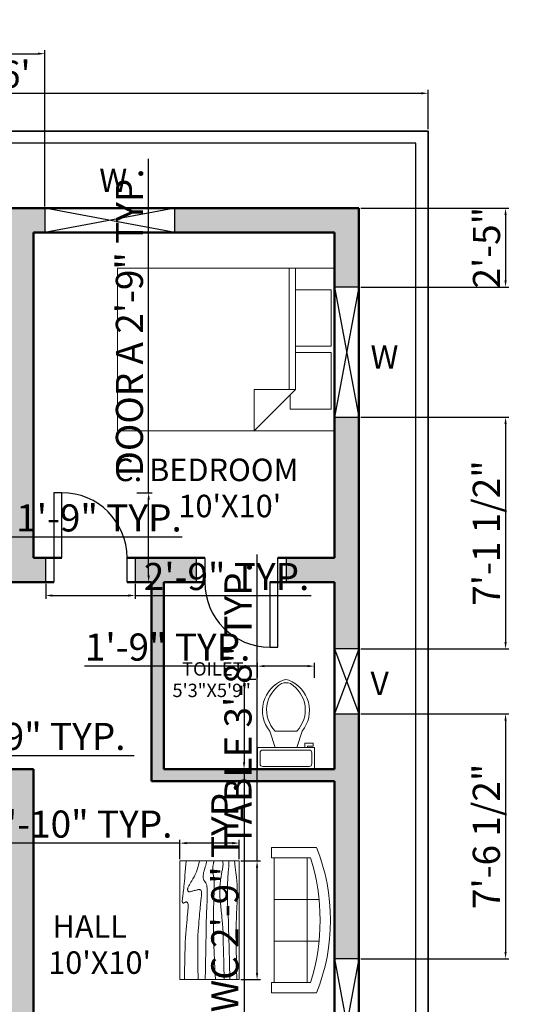
# Model space of a CAD drawing. Units: inches. Extents: x 2789 to 3623, y 2388 to 2993.
# Tile 5 of 5: x 3435 to 3623, y 2601 to 2964. Entities that reach past the tile are written whole.
import ezdxf

# ---------------------------------------------------------------- set-up
doc = ezdxf.new("R2010")
doc.units = ezdxf.units.IN
for name, color, linetype, lineweight in [('A-ANNO-DIMS', 2, 'Continuous', 18), ('A-ANNO-TEXT', 7, 'Continuous', 18), ('A-AREA-IDEN', 7, 'Continuous', 18), ('A-FLOR-FIXT', 9, 'Continuous', 18), ('A-FURN', 8, 'Continuous', 18), ('A-WALL', 7, 'Continuous', 50), ('A-WALL-PATT', 5, 'Continuous', 13), ('C-PROP', 7, 'Continuous', 35), ('d', 1, 'Continuous', 25), ('L-WALL', 7, 'Continuous', 25), ('v', 6, 'Continuous', 25), ('w', 170, 'Continuous', 25)]:
    doc.layers.add(name, color=color, linetype=linetype, lineweight=lineweight)
doc.styles.get("Standard").update_dxf_attribs({"font": 'arial.ttf'})
doc.dimstyles.new('ISO-25', dxfattribs={"dimtxt": 10, "dimasz": 2.5, "dimexe": 1.25, "dimexo": 0.625, "dimtad": 1, "dimlunit": 4, "dimtxsty": 'Standard', "dimcen": 2.5, "dimadec": 0, "dimazin": 0, "dimtfac": 1, "dimtmove": 0, "dimatfit": 3, "dimfxl": 1, "dimarcsym": 0})

# ---------------------------------------------------------------- blocks, each defined once
blk = doc.blocks.new('Sofa - Roundback 7 ft.')
for p, q in [((-12.00002, -32.4421), (-12.00003, -6.5971)), ((11.99997, -32.4421), (11.99998, -6.5971)), ((-36.000027, -34), (-36.000027, -11.4696)), ((-35.999844, -13.3819), (35.9998, -13.3819)), ((35.99998, -34), (35.99998, -11.4696)), ((-36.000027, -32.4421), (35.99998, -32.4421))]:
    blk.add_line(p, q)
for points in [[(-36.000027, -34), (-42.000027, -34), (-42.000027, -8)], [(41.99998, -8), (41.99998, -34), (35.99998, -34)]]:
    blk.add_lwpolyline(points)
for centre, radius, start, end in [((0, -114.25), 114.25, 68.43141, 111.5686), ((-0.00001, -127.1968), 121.1968, 72.72033, 107.2797)]:
    blk.add_arc(centre, radius, start, end)
blk = doc.blocks.new('Table - Rectangular Woodgrain 60 x 30 in.')
for p, q in [((0, 0), (0, -30)), ((60, 0), (0, 0)), ((60, -30), (60, 0)), ((0, -30), (60, -30))]:
    blk.add_line(p, q)
for points in [[(0, -2.4), (4.8155, -2.418), (9.0302, -2.4688), (12.709, -2.5477), (15.9167, -2.65), (18.7181, -2.7711), (21.1781, -2.9063), (23.3616, -3.0508), (25.3333, -3.2), (27.1477, -3.3495), (28.8172, -3.4958), (30.3437, -3.636), (31.7291, -3.7667), (32.9756, -3.8849), (34.0849, -3.9875), (35.059, -4.0714), (35.9, -4.1334), (36.6114, -4.1711), (37.2041, -4.1854), (37.6906, -4.1779), (38.0833, -4.15), (38.3948, -4.1034), (38.6375, -4.0396), (38.8239, -3.9602), (38.9666, -3.8667), (39.0764, -3.7608), (39.1573, -3.6448), (39.2116, -3.521), (39.2416, -3.3917), (39.2498, -3.2593), (39.2385, -3.1261), (39.21, -2.9944), (39.1666, -2.8667), (39.111, -2.7447), (39.0468, -2.6281), (38.978, -2.5163), (38.9083, -2.4083), (38.8418, -2.3035), (38.7823, -2.201), (38.7337, -2.1001), (38.7, -2), (38.6844, -1.9003), (38.6875, -1.8021), (38.7094, -1.707), (38.75, -1.6167), (38.8094, -1.5326), (38.8875, -1.4563), (38.9844, -1.3893), (39.1, -1.3333), (39.2351, -1.2896), (39.3937, -1.2583), (39.5804, -1.2396), (39.8, -1.2333), (40.057, -1.2396), (40.3562, -1.2583), (40.7023, -1.2896), (41.1, -1.3333), (41.5547, -1.3895), (42.0755, -1.4573), (42.6721, -1.5361), (43.3542, -1.625), (44.1316, -1.7233), (45.014, -1.8302), (46.0114, -1.9449), (47.1333, -2.0667), (48.3862, -2.1947), (49.7625, -2.3281), (51.2513, -2.4663), (52.8416, -2.6083), (54.5226, -2.7535), (56.2833, -2.9011), (58.1127, -3.0501), (60, -3.2)], [(0, -9.2), (6.5759, -9.0858), (11.9385, -9.0365), (16.2527, -9.0418), (19.6833, -9.0917), (22.3952, -9.1759), (24.5531, -9.2844), (26.322, -9.4069), (27.8666, -9.5333), (29.3241, -9.6553), (30.7203, -9.7719), (32.0532, -9.8837), (33.3208, -9.9917), (34.5213, -10.0965), (35.6526, -10.199), (36.7128, -10.2999), (37.7, -10.4), (38.6129, -10.4996), (39.4531, -10.5969), (40.223, -10.6895), (40.925, -10.775), (41.5613, -10.8512), (42.1344, -10.9156), (42.6465, -10.966), (43.1, -11), (43.4976, -11.0158), (43.8437, -11.0136), (44.143, -10.9942), (44.4, -10.9583), (44.6195, -10.9069), (44.8062, -10.8406), (44.9648, -10.7603), (45.1, -10.6667), (45.2155, -10.5598), (45.3114, -10.4365), (45.3871, -10.2929), (45.4416, -10.125), (45.4743, -9.929), (45.4844, -9.7011), (45.4709, -9.4371), (45.4333, -9.1333), (45.3716, -8.7883), (45.2896, -8.4104), (45.1919, -8.0107), (45.0833, -7.6), (44.9685, -7.1893), (44.8521, -6.7896), (44.7388, -6.4117), (44.6333, -6.0667), (44.54, -5.7628), (44.4614, -5.4979), (44.4001, -5.2675), (44.3583, -5.0667), (44.3384, -4.8909), (44.3427, -4.7354), (44.3736, -4.5956), (44.4333, -4.4667), (44.5236, -4.3453), (44.6427, -4.2333), (44.7884, -4.1339), (44.9583, -4.05), (45.1501, -3.9849), (45.3614, -3.9417), (45.59, -3.9234), (45.8333, -3.9333), (46.0915, -3.9749), (46.3734, -4.0531), (46.6906, -4.1736), (47.0542, -4.3417), (47.4756, -4.5629), (47.9661, -4.8427), (48.5372, -5.1866), (49.2, -5.6), (49.9676, -6.0844), (50.8594, -6.625), (51.8965, -7.2031), (53.1, -7.8), (54.491, -8.3969), (56.0906, -8.975), (57.9199, -9.5156), (60, -10)], [(0, -12.8), (5.1847, -12.9322), (9.6213, -13.0323), (13.3963, -13.1059), (16.5958, -13.1583), (19.3063, -13.1952), (21.614, -13.2219), (23.6054, -13.2439), (25.3666, -13.2667), (26.9728, -13.2947), (28.4531, -13.3281), (29.8256, -13.3663), (31.1083, -13.4083), (32.3191, -13.4535), (33.476, -13.501), (34.597, -13.5501), (35.7, -13.6), (36.7984, -13.6497), (37.8875, -13.6979), (38.9578, -13.743), (40, -13.7833), (41.0047, -13.8174), (41.9625, -13.8438), (42.864, -13.8607), (43.7, -13.8667), (44.4631, -13.8604), (45.1552, -13.8417), (45.7801, -13.8104), (46.3416, -13.7667), (46.8439, -13.7104), (47.2906, -13.6417), (47.6858, -13.5604), (48.0333, -13.4667), (48.3375, -13.3608), (48.6042, -13.2448), (48.8396, -13.121), (49.05, -12.9917), (49.2417, -12.8593), (49.4208, -12.7261), (49.5937, -12.5944), (49.7667, -12.4667), (49.9452, -12.3451), (50.1323, -12.2313), (50.3303, -12.1268), (50.5416, -12.0333), (50.7686, -11.9524), (51.0135, -11.8854), (51.2788, -11.8341), (51.5666, -11.8), (51.8785, -11.7843), (52.2116, -11.7865), (52.562, -11.8059), (52.926, -11.8417), (53.2998, -11.8931), (53.6795, -11.9594), (54.0614, -12.0397), (54.4416, -12.1333), (54.8223, -12.2401), (55.2293, -12.3625), (55.6942, -12.5037), (56.2489, -12.6667), (56.9251, -12.8547), (57.7545, -13.0708), (58.7689, -13.3182), (60, -13.6)], [(0, -18), (5.124, -17.7273), (9.6609, -17.5057), (13.6705, -17.3303), (17.2125, -17.1958), (20.3467, -17.0973), (23.1328, -17.0297), (25.6307, -16.9878), (27.9, -16.9667), (29.9928, -16.9617), (31.9302, -16.9703), (33.7254, -16.9907), (35.3917, -17.0208), (36.9423, -17.0588), (38.3906, -17.1026), (39.7499, -17.1503), (41.0333, -17.2), (42.2519, -17.2496), (43.4073, -17.2969), (44.4986, -17.3395), (45.525, -17.375), (46.4858, -17.4012), (47.3802, -17.4156), (48.2074, -17.416), (48.9667, -17.4), (49.6583, -17.3662), (50.2872, -17.3167), (50.8595, -17.2547), (51.3812, -17.1833), (51.8584, -17.1057), (52.2971, -17.025), (52.7034, -16.9443), (53.0833, -16.8667), (53.443, -16.7951), (53.789, -16.7313), (54.128, -16.6768), (54.4666, -16.6334), (54.8115, -16.6024), (55.1693, -16.5854), (55.5465, -16.5841), (55.95, -16.6), (56.3828, -16.6337), (56.8346, -16.6823), (57.2915, -16.7418), (57.7396, -16.8084), (58.165, -16.878), (58.5539, -16.9469), (58.8924, -17.0111), (59.1666, -17.0667), (59.3679, -17.1107), (59.5078, -17.1438), (59.6032, -17.1675), (59.6708, -17.1833), (59.7275, -17.193), (59.7901, -17.1979), (59.8753, -17.1998), (60, -17.2)], [(0, -22.4), (8.0098, -22.2501), (14.4094, -22.1011), (19.4168, -21.9535), (23.25, -21.8083), (26.1269, -21.6663), (28.2656, -21.5281), (29.884, -21.3947), (31.2, -21.2667), (32.3967, -21.1448), (33.5172, -21.0292), (34.5697, -20.9198), (35.5625, -20.8167), (36.5037, -20.7198), (37.4015, -20.6292), (38.2642, -20.5448), (39.1, -20.4667), (39.9164, -20.3951), (40.7187, -20.3313), (41.5117, -20.2768), (42.3, -20.2333), (43.0883, -20.2024), (43.8812, -20.1854), (44.6836, -20.1841), (45.5, -20.2), (46.3328, -20.234), (47.1747, -20.2844), (48.0163, -20.3488), (48.8479, -20.425), (49.66, -20.5106), (50.4429, -20.6031), (51.1872, -20.7004), (51.8833, -20.8), (52.5246, -20.8999), (53.1166, -20.9995), (53.6681, -21.0983), (54.1875, -21.1958), (54.6834, -21.2919), (55.1646, -21.3859), (55.6394, -21.4777), (56.1167, -21.5667), (56.6028, -21.6515), (57.0961, -21.7266), (57.5929, -21.7852), (58.0896, -21.8208), (58.5823, -21.8268), (59.0674, -21.7964), (59.5412, -21.723), (60, -21.6)], [(0, -25.2), (8.6355, -25.0504), (15.7026, -24.9031), (21.4049, -24.7606), (25.9458, -24.625), (29.529, -24.4988), (32.3578, -24.3844), (34.6359, -24.284), (36.5667, -24.2), (38.3213, -24.1341), (39.9417, -24.0854), (41.437, -24.0523), (42.8167, -24.0333), (44.0901, -24.0268), (45.2667, -24.0313), (46.3557, -24.0451), (47.3667, -24.0667), (48.309, -24.0947), (49.1928, -24.1287), (50.0284, -24.168), (50.826, -24.2125), (51.5959, -24.2617), (52.3483, -24.3151), (53.0935, -24.3725), (53.8417, -24.4334), (54.6009, -24.497), (55.3699, -24.561), (56.1454, -24.6226), (56.9239, -24.6792), (57.7021, -24.7279), (58.4764, -24.7662), (59.2435, -24.7911), (60, -24.8)], [(0, -28.8), (5.6867, -28.6681), (10.45, -28.5698), (14.407, -28.5012), (17.675, -28.4584), (20.3711, -28.4374), (22.6125, -28.4344), (24.5164, -28.4455), (26.2, -28.4667), (27.762, -28.4947), (29.2276, -28.5281), (30.6033, -28.5663), (31.8958, -28.6084), (33.1118, -28.6535), (34.2578, -28.7011), (35.3405, -28.7501), (36.3666, -28.8), (37.3443, -28.8497), (38.288, -28.8974), (39.2137, -28.9412), (40.1375, -28.9792), (41.0753, -29.0093), (42.0432, -29.0297), (43.0572, -29.0384), (44.1333, -29.0333), (45.2936, -29.0114), (46.5843, -28.9641), (48.0579, -28.8816), (49.7666, -28.7542), (51.7629, -28.5721), (54.0989, -28.3255), (56.8272, -28.0048), (60, -27.6)]]:
    blk.add_lwpolyline(points)
blk = doc.blocks.new('Toilet - top')
for p, q in [((9.5, -6), (9.5, -2)), ((-10, -8.5), (-8, -8.5)), ((-10, -9.5), (-10, -8.5)), ((-7, -9.5), (-10, -9.5)), ((-8, -8.5), (-8, -8)), ((-7, -8), (-7, -9.5)), ((-4, -8), (-6, -14)), ((4, -8), (6, -14)), ((4, -14), (-4, -14))]:
    blk.add_line(p, q)
blk.add_lwpolyline([(10.5, -8), (10.5, 0), (-10.5, 0), (-10.5, -8)], close=True)
for points in [[(-9.5, -2), (-9.5, -6)], [(8.5, -1), (-8.5, -1)], [(-8.5, -7), (8.5, -7)]]:
    blk.add_lwpolyline(points)
for centre, radius, start, end in [((-8.62, -1.88), 0.884, 81.8699, 188.1301), ((8.62, -1.88), 0.884, 351.8699, 98.1301), ((-8.62, -6.12), 0.884, 171.8699, 278.1301), ((8.62, -6.12), 0.884, 261.8699, 8.1301), ((3.52, -21.58), 12.17, 141.4691, 247.9714), ((4.2, -21.82), 11.33, 136.3677, 238.9468), ((-3.52, -21.58), 12.17, 292.0284, 38.5307), ((-4.2, -21.82), 11.33, 301.053, 43.6321), ((0, -27.88), 4, 245.7318, 294.2682), ((0, -29), 4, 254.8605, 285.1395)]:
    blk.add_arc(centre, radius, start, end)
blk = doc.blocks.new('Bed - Queen')
for p, q in [((0, -80.00003), (0, 0)), ((0, 0), (59.99999, 0)), ((59.99999, 0), (59.99999, -80.00003)), ((7.99999, -1.2), (28.79998, -1.2)), ((7.99999, -14.4), (7.99999, -1.2)), ((28.79998, -1.2), (28.79998, -14.4)), ((31.19999, -1.2), (51.99999, -1.2)), ((31.19999, -14.4), (31.19999, -1.2)), ((51.99999, -1.2), (51.99999, -16.4)), ((0, -14.4), (44.8, -14.4)), ((59.99999, -29.6), (44.8, -14.4)), ((44.8, -14.4), (44.8, -29.6)), ((44.8, -16.8), (0, -16.8)), ((51.99999, -16.4), (46.79936, -16.4)), ((44.8, -29.6), (59.99999, -29.6)), ((59.99999, -80.00003), (0, -80.00003))]:
    blk.add_line(p, q)
blk = doc.blocks.new('*D14')
at = {"layer": 'A-ANNO-DIMS', "color": 0, "lineweight": -2, "transparency": 16777216}
for p, q in [((3273.51, 2923.47), (3273.51, 2938.03)), ((3276.01, 2936.78), (3583.01, 2936.78)), ((3585.51, 2923.47), (3585.51, 2938.03))]:
    blk.add_line(p, q, dxfattribs=at)
at = {"layer": 'A-ANNO-DIMS', "color": 0, "transparency": 16777216}
for points in [[(3276.01, 2937.19), (3276.01, 2936.36), (3273.51, 2936.78)], [(3583.01, 2937.19), (3583.01, 2936.36), (3585.51, 2936.78)]]:
    blk.add_solid(points, dxfattribs=at)
at = {"layer": 'Defpoints', "color": 0, "transparency": 16777216}
for p in [(3585.51, 2936.78), (3273.51, 2922.84), (3585.51, 2922.84)]:
    blk.add_point(p, dxfattribs=at)
at = {"layer": 'A-ANNO-DIMS', "color": 0, "transparency": 16777216, "insert": (3429.51, 2942.51), "char_height": 10, "attachment_point": 5}
blk.add_mtext("26'", dxfattribs=at)
blk = doc.blocks.new('DOOR-24IN-JAMB-9IN')
for points in [[(0, 24), (-3, 24), (-3, 0), (0, 0)], [(-6, 0), (-3, 0), (-3, -9), (-6, -9)], [(24, 0), (27, 0), (27, -9), (24, -9)]]:
    blk.add_lwpolyline(points, close=True)
blk.add_arc((0, 0), 24, 0, 90)
blk = doc.blocks.new('WINDOW-48IN')
for p, q in [((48, 9), (0, 0)), ((48, 0), (0, 9))]:
    blk.add_line(p, q)
blk.add_lwpolyline([(0, 9), (0, 0), (48, 0), (48, 9)], close=True)
blk = doc.blocks.new('VENT-24IN')
for p, q in [((0, 24), (9, 0)), ((9, 24), (0, 0))]:
    blk.add_line(p, q)
blk.add_lwpolyline([(0, 0), (9, 0), (9, 24), (0, 24)], close=True)
blk = doc.blocks.new('*D22')
at = {"layer": 'A-ANNO-DIMS', "color": 0, "lineweight": -2, "transparency": 16777216}
for p, q in [((3482.46, 2789.34), (3482.46, 2912.54)), ((3478.13, 2789.34), (3483.71, 2789.34)), ((3482.46, 2758.84), (3482.46, 2786.84)), ((3478.13, 2756.34), (3483.71, 2756.34))]:
    blk.add_line(p, q, dxfattribs=at)
at = {"layer": 'A-ANNO-DIMS', "color": 0, "transparency": 16777216}
for points in [[(3482.04, 2786.84), (3482.87, 2786.84), (3482.46, 2789.34)], [(3482.04, 2758.84), (3482.87, 2758.84), (3482.46, 2756.34)]]:
    blk.add_solid(points, dxfattribs=at)
at = {"layer": 'Defpoints', "color": 0, "transparency": 16777216}
for p in [(3477.51, 2789.34), (3482.46, 2789.34), (3477.51, 2756.34)]:
    blk.add_point(p, dxfattribs=at)
at = {"layer": 'A-ANNO-DIMS', "color": 0, "transparency": 16777216, "insert": (3476.66, 2852.19), "char_height": 10, "attachment_point": 5, "rotation": 90}
blk.add_mtext('DOOR A 2\'-9" TYP.', dxfattribs=at)
blk = doc.blocks.new('*D23')
at = {"layer": 'A-ANNO-DIMS', "color": 0, "lineweight": -2, "transparency": 16777216}
for p, q in [((3444.51, 2755.72), (3444.51, 2750.14)), ((3477.51, 2755.72), (3477.51, 2750.14)), ((3447.01, 2751.39), (3475.01, 2751.39)), ((3477.51, 2751.39), (3542.38, 2751.39))]:
    blk.add_line(p, q, dxfattribs=at)
at = {"layer": 'A-ANNO-DIMS', "color": 0, "transparency": 16777216}
for points in [[(3447.01, 2751.81), (3447.01, 2750.98), (3444.51, 2751.39)], [(3475.01, 2751.81), (3475.01, 2750.98), (3477.51, 2751.39)]]:
    blk.add_solid(points, dxfattribs=at)
at = {"layer": 'Defpoints', "color": 0, "transparency": 16777216}
for p in [(3444.51, 2756.34), (3477.51, 2756.34), (3477.51, 2751.39)]:
    blk.add_point(p, dxfattribs=at)
at = {"layer": 'A-ANNO-DIMS', "color": 0, "transparency": 16777216, "insert": (3511.19, 2757.12), "char_height": 10, "attachment_point": 5}
blk.add_mtext('2\'-9" TYP.', dxfattribs=at)
blk = doc.blocks.new('*D31')
at = {"layer": 'A-ANNO-DIMS', "color": 0, "lineweight": -2, "transparency": 16777216}
for p, q in [((3410.01, 2777.79), (3410.01, 2771.76)), ((3431.01, 2777.79), (3431.01, 2771.76)), ((3412.51, 2773.01), (3428.51, 2773.01)), ((3431.01, 2773.01), (3494.78, 2773.01))]:
    blk.add_line(p, q, dxfattribs=at)
at = {"layer": 'A-ANNO-DIMS', "color": 0, "transparency": 16777216}
for points in [[(3412.51, 2773.43), (3412.51, 2772.59), (3410.01, 2773.01)], [(3428.51, 2773.43), (3428.51, 2772.59), (3431.01, 2773.01)]]:
    blk.add_solid(points, dxfattribs=at)
at = {"layer": 'Defpoints', "color": 0, "transparency": 16777216}
for p in [(3410.01, 2778.41), (3431.01, 2778.41), (3431.01, 2773.01)]:
    blk.add_point(p, dxfattribs=at)
at = {"layer": 'A-ANNO-DIMS', "color": 0, "transparency": 16777216, "insert": (3464.15, 2778.74), "char_height": 10, "attachment_point": 5}
blk.add_mtext('1\'-9" TYP.', dxfattribs=at)
blk = doc.blocks.new('*D34')
at = {"layer": 'A-ANNO-DIMS', "color": 0, "lineweight": -2, "transparency": 16777216}
for p, q in [((3522.44, 2653.44), (3522.44, 2766.54)), ((3516.49, 2653.44), (3523.69, 2653.44)), ((3522.44, 2612.13), (3522.44, 2650.94)), ((3516.49, 2609.63), (3523.69, 2609.63))]:
    blk.add_line(p, q, dxfattribs=at)
at = {"layer": 'A-ANNO-DIMS', "color": 0, "transparency": 16777216}
for points in [[(3522.02, 2650.94), (3522.85, 2650.94), (3522.44, 2653.44)], [(3522.02, 2612.13), (3522.85, 2612.13), (3522.44, 2609.63)]]:
    blk.add_solid(points, dxfattribs=at)
at = {"layer": 'Defpoints', "color": 0, "transparency": 16777216}
for p in [(3515.86, 2653.44), (3522.44, 2653.44), (3515.86, 2609.63)]:
    blk.add_point(p, dxfattribs=at)
at = {"layer": 'A-ANNO-DIMS', "color": 0, "transparency": 16777216, "insert": (3516.7, 2711.24), "char_height": 10, "attachment_point": 5, "rotation": 90}
blk.add_mtext('TABLE 3\'-8" TYP.', dxfattribs=at)
blk = doc.blocks.new('*D35')
at = {"layer": 'A-ANNO-DIMS', "color": 0, "lineweight": -2, "transparency": 16777216}
for p, q in [((3493.96, 2654.07), (3493.96, 2661.26)), ((3515.86, 2654.07), (3515.86, 2661.26)), ((3493.96, 2660.01), (3422.42, 2660.01)), ((3513.36, 2660.01), (3496.46, 2660.01))]:
    blk.add_line(p, q, dxfattribs=at)
at = {"layer": 'A-ANNO-DIMS', "color": 0, "transparency": 16777216}
for points in [[(3496.46, 2660.43), (3496.46, 2659.6), (3493.96, 2660.01)], [(3513.36, 2660.43), (3513.36, 2659.6), (3515.86, 2660.01)]]:
    blk.add_solid(points, dxfattribs=at)
at = {"layer": 'Defpoints', "color": 0, "transparency": 16777216}
for p in [(3493.96, 2660.01), (3493.96, 2653.44), (3515.86, 2653.44)]:
    blk.add_point(p, dxfattribs=at)
at = {"layer": 'A-ANNO-DIMS', "color": 0, "transparency": 16777216, "insert": (3456.94, 2665.74), "char_height": 10, "attachment_point": 5}
blk.add_mtext('1\'-10" TYP.', dxfattribs=at)
blk = doc.blocks.new('*D36')
at = {"layer": 'A-ANNO-DIMS', "color": 0, "lineweight": -2, "transparency": 16777216}
for p, q in [((3521.97, 2720.39), (3516.39, 2720.39)), ((3517.64, 2717.89), (3517.64, 2689.84)), ((3521.97, 2687.34), (3516.39, 2687.34)), ((3517.64, 2687.34), (3517.64, 2595.07))]:
    blk.add_line(p, q, dxfattribs=at)
at = {"layer": 'A-ANNO-DIMS', "color": 0, "transparency": 16777216}
for points in [[(3517.22, 2717.89), (3518.06, 2717.89), (3517.64, 2720.39)], [(3517.22, 2689.84), (3518.06, 2689.84), (3517.64, 2687.34)]]:
    blk.add_solid(points, dxfattribs=at)
at = {"layer": 'Defpoints', "color": 0, "transparency": 16777216}
for p in [(3522.6, 2720.39), (3517.64, 2687.34), (3522.6, 2687.34)]:
    blk.add_point(p, dxfattribs=at)
at = {"layer": 'A-ANNO-DIMS', "color": 0, "transparency": 16777216, "insert": (3511.84, 2639.96), "char_height": 10, "attachment_point": 5, "rotation": 90}
blk.add_mtext('WC 2\'-9" TYP.', dxfattribs=at)
blk = doc.blocks.new('*D37')
at = {"layer": 'A-ANNO-DIMS', "color": 0, "lineweight": -2, "transparency": 16777216}
for p, q in [((3522.6, 2721.01), (3522.6, 2726.59)), ((3543.6, 2721.01), (3543.6, 2726.59)), ((3522.6, 2725.34), (3458.83, 2725.34)), ((3541.1, 2725.34), (3525.1, 2725.34))]:
    blk.add_line(p, q, dxfattribs=at)
at = {"layer": 'A-ANNO-DIMS', "color": 0, "transparency": 16777216}
for points in [[(3525.1, 2725.76), (3525.1, 2724.93), (3522.6, 2725.34)], [(3541.1, 2725.76), (3541.1, 2724.93), (3543.6, 2725.34)]]:
    blk.add_solid(points, dxfattribs=at)
at = {"layer": 'Defpoints', "color": 0, "transparency": 16777216}
for p in [(3522.6, 2725.34), (3522.6, 2720.39), (3543.6, 2720.39)]:
    blk.add_point(p, dxfattribs=at)
at = {"layer": 'A-ANNO-DIMS', "color": 0, "transparency": 16777216, "insert": (3489.46, 2731.08), "char_height": 10, "attachment_point": 5}
blk.add_mtext('1\'-9" TYP.', dxfattribs=at)
blk = doc.blocks.new('*D38')
at = {"layer": 'A-ANNO-DIMS', "color": 0, "lineweight": -2, "transparency": 16777216}
for p, q in [((3320.88, 2687.97), (3320.88, 2693.54)), ((3353.88, 2687.97), (3353.88, 2693.54)), ((3323.38, 2692.29), (3351.38, 2692.29)), ((3353.88, 2692.29), (3477.08, 2692.29))]:
    blk.add_line(p, q, dxfattribs=at)
at = {"layer": 'A-ANNO-DIMS', "color": 0, "transparency": 16777216}
for points in [[(3323.38, 2692.71), (3323.38, 2691.88), (3320.88, 2692.29)], [(3351.38, 2692.71), (3351.38, 2691.88), (3353.88, 2692.29)]]:
    blk.add_solid(points, dxfattribs=at)
at = {"layer": 'Defpoints', "color": 0, "transparency": 16777216}
for p in [(3353.88, 2692.29), (3320.88, 2687.34), (3353.88, 2687.34)]:
    blk.add_point(p, dxfattribs=at)
at = {"layer": 'A-ANNO-DIMS', "color": 0, "transparency": 16777216, "insert": (3416.73, 2698.09), "char_height": 10, "attachment_point": 5}
blk.add_mtext('DOOR B 2\'-9" TYP.', dxfattribs=at)
blk = doc.blocks.new('*D51')
at = {"layer": 'A-ANNO-DIMS', "color": 0, "lineweight": -2, "transparency": 16777216}
for p, q in [((3363.15, 2894.97), (3363.15, 2952.64)), ((3365.65, 2951.39), (3441.65, 2951.39)), ((3444.15, 2894.97), (3444.15, 2952.64))]:
    blk.add_line(p, q, dxfattribs=at)
at = {"layer": 'A-ANNO-DIMS', "color": 0, "transparency": 16777216}
for points in [[(3365.65, 2951.81), (3365.65, 2950.98), (3363.15, 2951.39)], [(3441.65, 2951.81), (3441.65, 2950.98), (3444.15, 2951.39)]]:
    blk.add_solid(points, dxfattribs=at)
at = {"layer": 'Defpoints', "color": 0, "transparency": 16777216}
for p in [(3444.15, 2951.39), (3363.15, 2894.34), (3444.15, 2894.34)]:
    blk.add_point(p, dxfattribs=at)
at = {"layer": 'A-ANNO-DIMS', "color": 0, "transparency": 16777216, "insert": (3403.65, 2957.12), "char_height": 10, "attachment_point": 5}
blk.add_mtext('6\'-9"', dxfattribs=at)
blk = doc.blocks.new('*D54')
at = {"layer": 'A-ANNO-DIMS', "color": 0, "lineweight": -2, "transparency": 16777216}
for p, q in [((3560.64, 2894.34), (3615.31, 2894.34)), ((3614.06, 2891.84), (3614.06, 2867.73)), ((3560.64, 2865.23), (3615.31, 2865.23))]:
    blk.add_line(p, q, dxfattribs=at)
at = {"layer": 'A-ANNO-DIMS', "color": 0, "transparency": 16777216}
for points in [[(3613.65, 2891.84), (3614.48, 2891.84), (3614.06, 2894.34)], [(3613.65, 2867.73), (3614.48, 2867.73), (3614.06, 2865.23)]]:
    blk.add_solid(points, dxfattribs=at)
at = {"layer": 'Defpoints', "color": 0, "transparency": 16777216}
for p in [(3560.01, 2894.34), (3560.01, 2865.23), (3614.06, 2865.23)]:
    blk.add_point(p, dxfattribs=at)
at = {"layer": 'A-ANNO-DIMS', "color": 0, "transparency": 16777216, "insert": (3608.33, 2879.79), "char_height": 10, "attachment_point": 5, "rotation": 90}
blk.add_mtext('2\'-5"', dxfattribs=at)
blk = doc.blocks.new('*D55')
at = {"layer": 'A-ANNO-DIMS', "color": 0, "lineweight": -2, "transparency": 16777216}
for p, q in [((3560.64, 2817.23), (3615.31, 2817.23)), ((3614.06, 2814.73), (3614.06, 2734.21)), ((3560.64, 2731.71), (3615.31, 2731.71))]:
    blk.add_line(p, q, dxfattribs=at)
at = {"layer": 'A-ANNO-DIMS', "color": 0, "transparency": 16777216}
for points in [[(3613.65, 2814.73), (3614.48, 2814.73), (3614.06, 2817.23)], [(3613.65, 2734.21), (3614.48, 2734.21), (3614.06, 2731.71)]]:
    blk.add_solid(points, dxfattribs=at)
at = {"layer": 'Defpoints', "color": 0, "transparency": 16777216}
for p in [(3560.01, 2817.23), (3560.01, 2731.71), (3614.06, 2731.71)]:
    blk.add_point(p, dxfattribs=at)
at = {"layer": 'A-ANNO-DIMS', "color": 0, "transparency": 16777216, "insert": (3608.27, 2774.47), "char_height": 10, "attachment_point": 5, "rotation": 90}
blk.add_mtext('7\'-1 1/2"', dxfattribs=at)
blk = doc.blocks.new('*D56')
at = {"layer": 'A-ANNO-DIMS', "color": 0, "lineweight": -2, "transparency": 16777216}
for p, q in [((3560.64, 2707.71), (3615.31, 2707.71)), ((3614.06, 2705.21), (3614.06, 2619.82)), ((3560.64, 2617.32), (3615.31, 2617.32))]:
    blk.add_line(p, q, dxfattribs=at)
at = {"layer": 'A-ANNO-DIMS', "color": 0, "transparency": 16777216}
for points in [[(3613.65, 2705.21), (3614.48, 2705.21), (3614.06, 2707.71)], [(3613.65, 2619.82), (3614.48, 2619.82), (3614.06, 2617.32)]]:
    blk.add_solid(points, dxfattribs=at)
at = {"layer": 'Defpoints', "color": 0, "transparency": 16777216}
for p in [(3560.01, 2707.71), (3560.01, 2617.32), (3614.06, 2617.32)]:
    blk.add_point(p, dxfattribs=at)
at = {"layer": 'A-ANNO-DIMS', "color": 0, "transparency": 16777216, "insert": (3608.27, 2662.51), "char_height": 10, "attachment_point": 5, "rotation": 90}
blk.add_mtext('7\'-6 1/2"', dxfattribs=at)

msp = doc.modelspace()

# ---------------------------------------------------------------- hatches: boundary and pattern name
at = {"layer": 'A-WALL-PATT'}
h = msp.add_hatch(color=256, dxfattribs=at)
h.dxf.hatch_style = 1
h.paths.add_polyline_path([(3560.015, 2707.71), (3551.015, 2707.71), (3551.015, 2687.342), (3488.015, 2687.342), (3488.015, 2756.342), (3500.148, 2756.342), (3500.148, 2765.342), (3477.506, 2765.342), (3477.506, 2756.342), (3483.515, 2756.342), (3483.515, 2682.842), (3551.015, 2682.842), (3551.015, 2617.319), (3560.015, 2617.319)])
h.paths.add_polyline_path([(3560.015, 2817.229), (3551.015, 2817.229), (3551.015, 2812.239), (3551.015, 2765.342), (3533.148, 2765.342), (3533.148, 2756.342), (3551.015, 2756.342), (3551.015, 2731.71), (3560.015, 2731.71)])
h.paths.add_polyline_path([(3560.015, 2894.342), (3492.148, 2894.342), (3492.148, 2885.342), (3551.015, 2885.342), (3551.015, 2865.229), (3560.015, 2865.229)])
h.paths.add_polyline_path([(3444.148, 2894.342), (3363.151, 2894.342), (3363.151, 2885.342), (3431.015, 2885.342), (3431.015, 2765.342), (3368.943, 2765.342), (3368.943, 2756.342), (3444.506, 2756.342), (3444.506, 2765.342), (3440.015, 2765.342), (3440.015, 2885.342), (3444.148, 2885.342)])
h.paths.add_polyline_path([(3311.015, 2885.342), (3315.151, 2885.342), (3315.151, 2894.342), (3302.015, 2894.342), (3302.015, 2819.267), (3311.015, 2819.267)])
h.paths.add_polyline_path([(3311.015, 2756.342), (3332.943, 2756.342), (3332.943, 2765.342), (3311.015, 2765.342), (3311.015, 2771.267), (3302.015, 2771.267), (3302.015, 2648.516), (3311.015, 2648.516), (3311.015, 2682.842), (3320.883, 2682.842), (3320.883, 2687.342), (3311.015, 2687.342)])
h.paths.add_polyline_path([(3439.015, 2489.342), (3311.015, 2489.342), (3311.015, 2553.842), (3317.302, 2553.842), (3317.302, 2562.842), (3311.015, 2562.842), (3311.015, 2600.516), (3302.015, 2600.516), (3302.015, 2480.342), (3439.015, 2480.342)])
h.paths.add_polyline_path([(3447.515, 2562.842), (3440.015, 2562.842), (3440.015, 2687.342), (3353.883, 2687.342), (3353.883, 2682.842), (3431.015, 2682.842), (3431.015, 2562.842), (3365.302, 2562.842), (3365.302, 2553.842), (3447.515, 2553.842)])
h.paths.add_polyline_path([(3560.015, 2569.319), (3551.015, 2569.319), (3551.015, 2562.842), (3541.085, 2562.842), (3541.085, 2553.842), (3560.015, 2553.842)])
h.paths.add_polyline_path([(3439.015, 2523.092), (3359.015, 2523.092), (3359.015, 2520.092), (3439.015, 2520.092)], flags=17)
h.paths.add_polyline_path([(3341.726, 2503.274), (3341.726, 2543.14), (3329.011, 2543.14), (3329.011, 2503.274)], flags=25)
h.paths.add_polyline_path([(3328.42, 2497.829), (3328.42, 2542.718), (3315.535, 2542.718), (3315.535, 2497.829)], flags=25)
h.paths.add_polyline_path([(3476.819, 2492.441), (3529.584, 2492.441), (3529.584, 2505.156), (3476.819, 2505.156)], flags=9)
h.paths.add_polyline_path([(3482.427, 2505.748), (3529.241, 2505.748), (3529.241, 2518.633), (3482.427, 2518.633)], flags=9)
h.paths.add_polyline_path([(3491.312, 2778.023), (3533.511, 2778.023), (3533.511, 2790.738), (3491.312, 2790.738)], flags=9)
h.paths.add_polyline_path([(3467.584, 2791.33), (3549.839, 2791.33), (3549.839, 2804.214), (3467.584, 2804.214)], flags=9)
h.paths.add_polyline_path([(3489.974, 2712.567), (3519.954, 2712.567), (3519.954, 2720.13), (3489.974, 2720.13)], flags=25)
h.paths.add_polyline_path([(3493.529, 2720.481), (3522.128, 2720.481), (3522.128, 2728.14), (3493.529, 2728.14)], flags=25)
h.paths.add_polyline_path([(3443.312, 2609.496), (3485.511, 2609.496), (3485.511, 2622.211), (3443.312, 2622.211)], flags=9)
h.paths.add_polyline_path([(3444.938, 2623.016), (3478.097, 2623.016), (3478.097, 2635.468), (3444.938, 2635.468)], flags=9)
h.paths.add_polyline_path([(3353.282, 2645.374), (3395.481, 2645.374), (3395.481, 2658.089), (3353.282, 2658.089)], flags=9)
h.paths.add_polyline_path([(3347.837, 2658.68), (3428.155, 2658.68), (3428.155, 2671.565), (3347.837, 2671.565)], flags=9)
h.paths.add_polyline_path([(3345.461, 2717.778), (3391.776, 2717.778), (3391.776, 2730.493), (3345.461, 2730.493)], flags=9)
h.paths.add_polyline_path([(3340.017, 2731.086), (3399.739, 2731.086), (3399.739, 2743.962), (3340.017, 2743.962)], flags=9)
h.paths.add_polyline_path([(3345.461, 2806.621), (3387.66, 2806.621), (3387.66, 2819.336), (3345.461, 2819.336)], flags=9)
h.paths.add_polyline_path([(3340.017, 2819.929), (3398.431, 2819.929), (3398.431, 2832.806), (3340.017, 2832.806)], flags=9)

# ---------------------------------------------------------------- linework, layer by layer
at = {"layer": 'A-WALL'}
for p, q in [((3560.015, 2894.342), (3302.015, 2894.342)), ((3560.015, 2480.342), (3560.015, 2894.342)), ((3551.015, 2885.342), (3440.015, 2885.342)), ((3440.015, 2885.342), (3440.015, 2765.342)), ((3551.015, 2765.342), (3551.015, 2885.342)), ((3450.506, 2765.342), (3440.015, 2765.342)), ((3503.148, 2765.342), (3474.506, 2765.342)), ((3551.015, 2765.342), (3530.148, 2765.342)), ((3447.506, 2756.342), (3368.943, 2756.342)), ((3483.515, 2756.342), (3474.506, 2756.342)), ((3483.515, 2682.842), (3483.515, 2756.342)), ((3488.015, 2687.342), (3488.015, 2756.342)), ((3503.148, 2756.342), (3488.015, 2756.342)), ((3551.015, 2756.342), (3527.148, 2756.342)), ((3551.015, 2687.342), (3551.015, 2756.342)), ((3440.015, 2687.342), (3350.883, 2687.342)), ((3440.015, 2687.342), (3440.015, 2562.842)), ((3551.015, 2687.342), (3488.015, 2687.342)), ((3551.015, 2682.842), (3483.515, 2682.842)), ((3551.015, 2562.842), (3551.015, 2682.842))]:
    msp.add_line(p, q, dxfattribs=at)
at = {"layer": 'C-PROP'}
msp.add_lwpolyline([(3273.515, 2442.842), (3585.515, 2442.842), (3585.515, 2922.842), (3273.515, 2922.842)], close=True, dxfattribs=at)
at = {"layer": 'L-WALL'}
for p, q in [((3581.015, 2918.342), (3278.015, 2918.342)), ((3581.015, 2447.342), (3581.015, 2918.342))]:
    msp.add_line(p, q, dxfattribs=at)

# ---------------------------------------------------------------- block references
at = {"layer": 'A-FLOR-FIXT', "rotation": 180}
msp.add_blockref('Toilet - top', (3533.096, 2687.342), dxfattribs=at)
at = {"layer": 'A-FURN', "rotation": 270}
msp.add_blockref('Bed - Queen', (3551.015, 2872.239), dxfattribs=at)
at = {"layer": 'A-FURN'}
for name, p, xscale, yscale, zscale, rotation in [('Sofa - Roundback 7 ft.', (3549.504, 2631.544), 0.639377291081551, 0.639377291081551, 0.639377291081551, 270), ('Table - Rectangular Woodgrain 60 x 30 in.', (3493.955, 2609.626), 0.7302634608291837, 0.7302634608291837, 0.7302634608291837, 90)]:
    msp.add_blockref(name, p, dxfattribs=dict(at, xscale=xscale, yscale=yscale, zscale=zscale, rotation=rotation))
at = {"layer": 'd'}
msp.add_blockref('DOOR-24IN-JAMB-9IN', (3450.506, 2765.342), dxfattribs=at)
at = {"layer": 'd', "rotation": 180}
msp.add_blockref('DOOR-24IN-JAMB-9IN', (3527.148, 2756.342), dxfattribs=at)
at = {"layer": 'v'}
msp.add_blockref('VENT-24IN', (3551.014, 2707.71), dxfattribs=at)
at = {"layer": 'w'}
msp.add_blockref('WINDOW-48IN', (3444.148, 2885.342), dxfattribs=at)
for p, rotation in [((3560.014, 2817.229), 90.00000000000225), ((3560.014, 2569.319), 90.00000000000207)]:
    msp.add_blockref('WINDOW-48IN', p, dxfattribs=dict(at, rotation=rotation))

# ---------------------------------------------------------------- texts
at = {"layer": 'A-ANNO-TEXT'}
for s, p in [('W', (3464.262, 2900.34)), ('W', (3564.263, 2835.179)), ('V', (3564.263, 2714.663))]:
    msp.add_text(s, height=8.603, dxfattribs=at).set_placement(p)
at = {"layer": 'A-AREA-IDEN'}
for s, height, p in [('C. BEDROOM ', 8.30108, (3469.732, 2793.619)), ("10'X10'", 8.3011, (3493.431, 2780.284)), ('TOILET ', 4.9345, (3494.806, 2721.842)), ('5\'3"X5\'9"', 4.9345, (3491.234, 2713.915)), ('HALL', 8.3011, (3447.014, 2625.092)), ("10'X10'", 8.3011, (3445.431, 2611.757))]:
    msp.add_text(s, height=height, dxfattribs=at).set_placement(p)

# ---------------------------------------------------------------- dimensions: what is measured, and where the dimension line sits
at = {"layer": 'A-ANNO-DIMS'}
for base, p1, p2, override, picture, middle in [((3444.148, 2951.392), (3363.151, 2894.342), (3444.148, 2894.342), {"dimdec": 1, "dimlfac": 1, "dimrnd": 0, "dimzin": 1, "dimdsep": 46, "dimlunit": 4, "dimfrac": 2}, '*D51', (3403.649, 2957.122)), ((3585.515, 2936.777), (3273.515, 2922.842), (3585.515, 2922.842), {"dimclrd": 0, "dimclre": 0, "dimclrt": 0}, '*D14', (3429.515, 2942.508))]:
    dim = msp.add_linear_dim(base=base, p1=p1, p2=p2, dimstyle='ISO-25', override=override, dxfattribs=at)
    dim.commit()
    dim.dimension.update_dxf_attribs({"geometry": picture, "text_midpoint": middle})
for base, p1, p2, angle, text, picture, middle in [((3482.456, 2789.342), (3477.506, 2756.342), (3477.506, 2789.342), 90, 'DOOR A <> TYP.', '*D22', (3476.657, 2852.19)), ((3522.435, 2653.442), (3515.863, 2609.626), (3515.863, 2653.442), 90, 'TABLE <> TYP.', '*D34', (3516.701, 2711.239)), ((3522.596, 2725.345), (3543.596, 2720.388), (3522.596, 2720.388), 180, '<> TYP.', '*D37', (3489.464, 2731.076)), ((3517.639, 2687.342), (3522.596, 2720.388), (3522.596, 2687.342), 270, 'WC <> TYP.', '*D36', (3511.844, 2639.957)), ((3493.955, 2660.014), (3515.863, 2653.442), (3493.955, 2653.442), 180, '<> TYP.', '*D35', (3456.939, 2665.745))]:
    dim = msp.add_linear_dim(base=base, p1=p1, p2=p2, angle=angle, text=text, dimstyle='ISO-25', override={"dimdec": 1, "dimlfac": 1, "dimrnd": 0, "dimzin": 1, "dimdsep": 46, "dimlunit": 4, "dimfrac": 2}, dxfattribs=at)
    dim.commit()
    dim.dimension.update_dxf_attribs({"geometry": picture, "text_midpoint": middle})
for base, p1, p2, picture, middle in [((3614.065, 2865.229), (3560.015, 2894.342), (3560.015, 2865.229), '*D54', (3608.334, 2879.785)), ((3614.065, 2731.71), (3560.015, 2817.229), (3560.015, 2731.71), '*D55', (3608.269, 2774.47)), ((3614.065, 2617.319), (3560.015, 2707.71), (3560.015, 2617.319), '*D56', (3608.269, 2662.515))]:
    dim = msp.add_linear_dim(base=base, p1=p1, p2=p2, angle=90, dimstyle='ISO-25', override={"dimdec": 1, "dimlfac": 1, "dimrnd": 0, "dimzin": 1, "dimdsep": 46, "dimlunit": 4, "dimfrac": 2}, dxfattribs=at)
    dim.commit()
    dim.dimension.update_dxf_attribs({"geometry": picture, "text_midpoint": middle})
for base, p1, p2, text, picture, middle in [((3431.015, 2773.011), (3410.015, 2778.411), (3431.015, 2778.411), '<> TYP.', '*D31', (3464.146, 2778.741)), ((3477.506, 2751.392), (3444.506, 2756.342), (3477.506, 2756.342), '<> TYP.', '*D23', (3511.194, 2757.122)), ((3353.883, 2692.292), (3320.883, 2687.342), (3353.883, 2687.342), 'DOOR B <> TYP.', '*D38', (3416.732, 2698.091))]:
    dim = msp.add_linear_dim(base=base, p1=p1, p2=p2, text=text, dimstyle='ISO-25', override={"dimdec": 1, "dimlfac": 1, "dimrnd": 0, "dimzin": 1, "dimdsep": 46, "dimlunit": 4, "dimfrac": 2}, dxfattribs=at)
    dim.commit()
    dim.dimension.update_dxf_attribs({"geometry": picture, "text_midpoint": middle})

doc.saveas('drawing.dxf')
